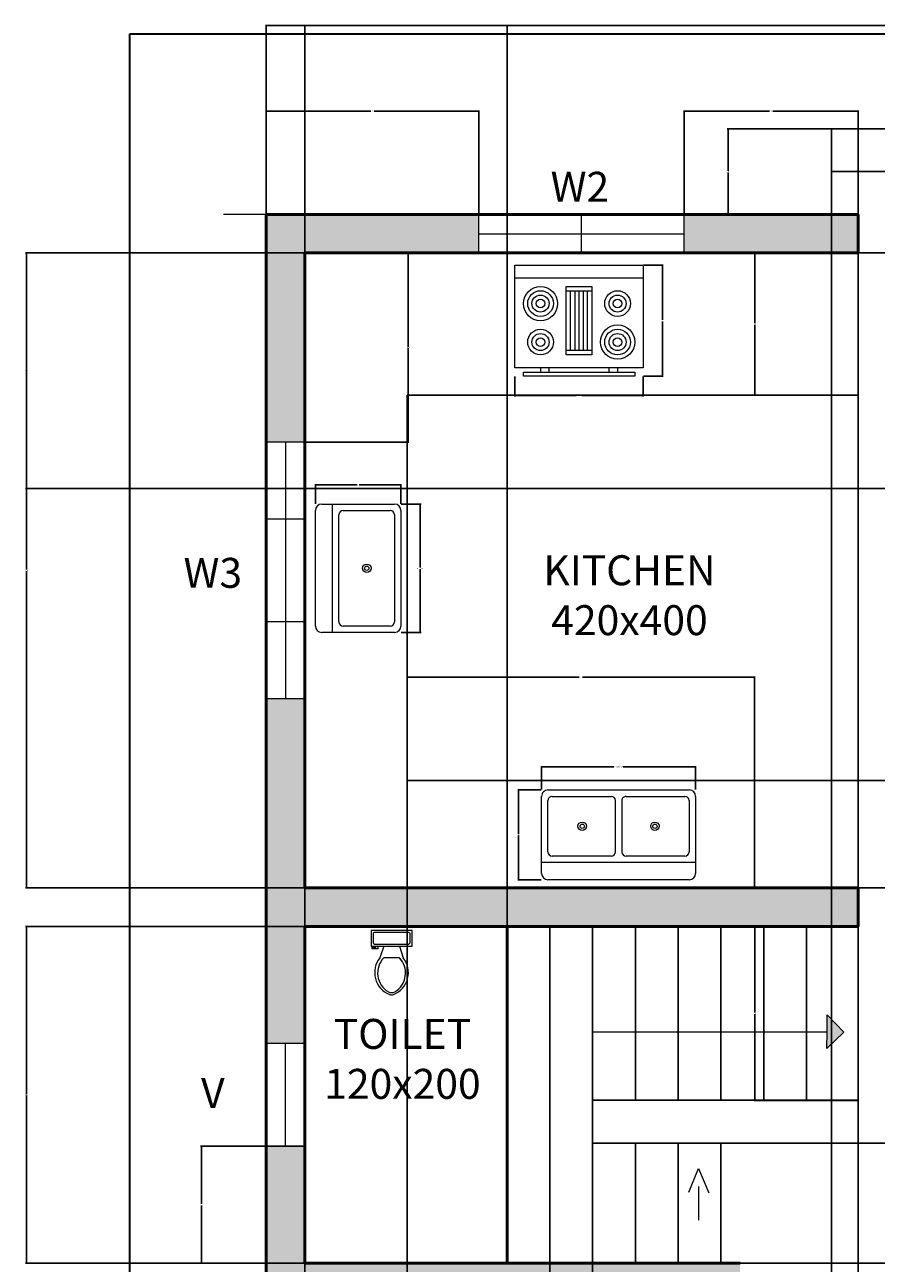
# Model space of a CAD drawing. Units: inches. Extents: x 5191 to 5616, y 7031 to 7539.
# Tile 3 of 4: x 5191 to 5390, y 7250 to 7539. Entities that reach past the tile are written whole.
import ezdxf

# ---------------------------------------------------------------- set-up
doc = ezdxf.new("R2010")
doc.units = ezdxf.units.IN
for name, color, linetype, lineweight in [('A-ANNO-DIMS', 2, 'Continuous', 13), ('A-ANNO-SYMB', 7, 'Continuous', 18), ('A-ANNO-TEXT', 7, 'Continuous', 18), ('A-ANNO-TTLB', 7, 'Continuous', 35), ('A-AREA-IDEN', 7, 'Continuous', 25), ('A-EQPM', 8, 'Continuous', 18), ('A-FLOR-CASE', 8, 'Continuous', 25), ('A-FLOR-FIXT', 9, 'Continuous', 18), ('A-FLOR-STRS', 7, 'Continuous', 25), ('A-GLAZ', 4, 'Continuous', 18), ('A-WALL', 7, 'Continuous', 50)]:
    doc.layers.add(name, color=color, linetype=linetype, lineweight=lineweight)
doc.layers.add('A-WALL-PATT', color=177, linetype='Continuous', lineweight=13, true_color=0x293189)
doc.styles.get("Standard").update_dxf_attribs({"font": 'arial.ttf'})
doc.dimstyles.get("Standard").update_dxf_attribs({"dimtxt": 0.18, "dimasz": 0.18, "dimexe": 0.18, "dimexo": 0.0625, "dimgap": 0.09, "dimtad": 0, "dimtih": 1, "dimtoh": 1, "dimdec": 4, "dimzin": 0, "dimdsep": 46, "dimtxsty": 'Standard', "dimcen": 0.09, "dimadec": 0, "dimazin": 0, "dimtfac": 1, "dimtdec": 4, "dimtofl": 0, "dimtmove": 0, "dimatfit": 3, "dimfxl": 1, "dimtolj": 1, "dimtzin": 0, "dimarcsym": 0})

# ---------------------------------------------------------------- blocks, each defined once
blk = doc.blocks.new('*U2')
for p, q in [((9.5, -6), (9.5, -2)), ((-10, -8.5), (-8, -8.5)), ((-10, -9.5), (-10, -8.5)), ((-7, -9.5), (-10, -9.5)), ((-8, -8.5), (-8, -8)), ((-7, -8), (-7, -9.5)), ((-4, -8), (-6, -14)), ((4, -8), (6, -14)), ((4, -14), (-4, -14))]:
    blk.add_line(p, q)
blk.add_lwpolyline([(10.5, -8), (10.5, 0), (-10.5, 0), (-10.5, -8)], close=True)
for points in [[(-9.5, -2), (-9.5, -6)], [(8.5, -1), (-8.5, -1)], [(-8.5, -7), (8.5, -7)]]:
    blk.add_lwpolyline(points)
for centre, radius, start, end in [((-8.62, -1.88), 0.884, 81.8699, 188.1301), ((-8.62, -6.12), 0.884, 171.8699, 278.1301), ((8.62, -1.88), 0.884, 351.8699, 98.1301), ((8.62, -6.12), 0.884, 261.8699, 8.1301), ((3.52, -21.58), 12.17, 141.46911, 247.97143), ((4.2, -21.82), 11.33, 136.36773, 238.94682), ((-3.52, -21.58), 12.17, 292.02843, 38.53071), ((-4.2, -21.82), 11.33, 301.05301, 43.63209), ((0, -27.88), 4, 245.73182, 294.26817), ((0, -29), 4, 254.86053, 285.13947)]:
    blk.add_arc(centre, radius, start, end)
blk = doc.blocks.new('Range-Oven - 30 in top')
for p, q in [((0, -3), (30, -3)), ((12, -6), (18, -6)), ((13, -20), (13, -6)), ((14, -6), (14, -20)), ((15, -20), (15, -6)), ((16, -6), (16, -20)), ((17, -20), (17, -6)), ((18, -20), (12, -20)), ((6, -24), (6, -25)), ((8, -25), (8, -24)), ((22, -25), (22, -24)), ((24, -24), (24, -25))]:
    blk.add_line(p, q)
for points in [[(0, -24), (0, 0), (30, 0), (30, -24)], [(12, -21), (12, -5), (18, -5), (18, -21)], [(2, -26), (2, -25), (28, -25), (28, -26)]]:
    blk.add_lwpolyline(points, close=True)
for centre, radius in [((6, -9), 4), ((6, -9), 3), ((6, -9), 2), ((6, -9), 1), ((24, -9), 3), ((24, -9), 2), ((24, -9), 1), ((24, -18), 4), ((6, -18), 3), ((6, -18), 2), ((6, -18), 1), ((24, -18), 3), ((24, -18), 2), ((24, -18), 1)]:
    blk.add_circle(centre, radius)
blk = doc.blocks.new('Sink-double - 36 in top')
for p, q in [((-18, -4), (18, -4)), ((-0.75, -18.5), (-0.75, -6.5)), ((0.75, -6.5), (0.75, -18.5))]:
    blk.add_line(p, q)
for points in [[(-16.5, 0), (16.5, 0)], [(-18, -19.5), (-18, -1.5)], [(18, -1.5), (18, -19.5)], [(-15.5, -5.5), (-1.75, -5.5)], [(1.75, -5.5), (15.5, -5.5)], [(-16.5, -18.5), (-16.5, -6.5)], [(16.5, -6.5), (16.5, -18.5)], [(-1.75, -19.5), (-15.5, -19.5)], [(15.5, -19.5), (1.75, -19.5)], [(16.5, -21), (-16.5, -21)]]:
    blk.add_lwpolyline(points)
for centre, radius in [((-8.5, -12.5), 1), ((8.5, -12.5), 1), ((-8.5, -12.5), 0.5), ((8.5, -12.5), 0.5)]:
    blk.add_circle(centre, radius)
for centre, radius, start, end in [((-16.5, -1.5), 1.5, 90, 180), ((16.5, -1.5), 1.5, 0, 90), ((-15.5, -6.5), 1, 90, 180), ((-1.75, -6.5), 1, 0, 90), ((1.75, -6.5), 1, 90, 180), ((15.5, -6.5), 1, 0, 90), ((-16.5, -19.5), 1.5, 180, 270), ((-15.5, -18.5), 1, 180, 270), ((-1.75, -18.5), 1, 270, 0), ((1.75, -18.5), 1, 180, 270), ((15.5, -18.5), 1, 270, 0), ((16.5, -19.5), 1.5, 270, 0)]:
    blk.add_arc(centre, radius, start, end)
blk = doc.blocks.new('Sink-single - 30 in top')
blk.add_line((-15, -3.999996), (15, -3.999996))
for points in [[(-13.5, 0), (13.5, 0)], [(-15, -18.499996), (-15, -1.5)], [(15, -1.5), (15, -18.499996)], [(-12.5, -5.499996), (12.5, -5.499996)], [(-13.5, -17.499996), (-13.5, -6.499996)], [(13.5, -6.499996), (13.5, -17.499996)], [(13.5, -19.999996), (-13.5, -19.999996)], [(12.5, -18.499996), (-12.5, -18.499996)]]:
    blk.add_lwpolyline(points)
for radius in [1, 0.5]:
    blk.add_circle((0, -11.999996), radius)
for centre, radius, start, end in [((-13.5, -1.5), 1.5, 90, 180), ((13.5, -1.5), 1.5, 0, 90), ((-12.5, -6.499996), 1, 90, 180), ((12.5, -6.499996), 1, 0, 90), ((-13.5, -18.499996), 1.5, 180, 270), ((-12.5, -17.499996), 1, 180, 270), ((12.5, -17.499996), 1, 270, 0), ((13.5, -18.499996), 1.5, 270, 0)]:
    blk.add_arc(centre, radius, start, end)
blk = doc.blocks.new('WIN-W2-48IN')
for p, q in [((0, 0), (0, 9)), ((24, 0), (24, 9)), ((48, 0), (48, 9)), ((0, 4.5), (48, 4.5))]:
    blk.add_line(p, q)
blk = doc.blocks.new('WIN-W3-60IN')
for p, q in [((9, 60), (0, 60)), ((4.5, 60), (4.5, 0)), ((9, 42), (0, 42)), ((9, 18), (0, 18)), ((9, 0), (0, 0))]:
    blk.add_line(p, q)
blk = doc.blocks.new('VENT-24IN')
for p, q in [((0, 0), (0, 9)), ((24, 0), (24, 9)), ((0, 4.5), (24, 4.5))]:
    blk.add_line(p, q)
blk = doc.blocks.new('*D25')
at = {"layer": 'A-ANNO-DIMS', "color": 0, "lineweight": -2, "transparency": 16777216}
for p, q in [((5305.74, 7456.87), (5305.74, 7452.25)), ((5335.74, 7456.87), (5335.74, 7452.25)), ((5305.92, 7452.43), (5320.05, 7452.43)), ((5335.56, 7452.43), (5321.44, 7452.43))]:
    blk.add_line(p, q, dxfattribs=at)
at = {"layer": 'A-ANNO-DIMS', "color": 0, "transparency": 16777216}
for points in [[(5305.92, 7452.46), (5305.92, 7452.4), (5305.74, 7452.43)], [(5335.56, 7452.46), (5335.56, 7452.4), (5335.74, 7452.43)]]:
    blk.add_solid(points, dxfattribs=at)
at = {"layer": 'Defpoints', "color": 0, "transparency": 16777216}
for p in [(5305.74, 7456.93), (5335.74, 7456.93), (5335.74, 7452.43)]:
    blk.add_point(p, dxfattribs=at)
at = {"layer": 'A-ANNO-DIMS', "color": 0, "transparency": 16777216, "insert": (5320.74, 7452.43), "char_height": 0.18, "attachment_point": 5}
blk.add_mtext('\\A1;RANGE 30', dxfattribs=at)
blk = doc.blocks.new('*D26')
at = {"layer": 'A-ANNO-DIMS', "color": 0, "lineweight": -2, "transparency": 16777216}
for p, q in [((5335.81, 7482.93), (5340.42, 7482.93)), ((5340.24, 7482.75), (5340.24, 7470.12)), ((5340.24, 7457.11), (5340.24, 7469.75)), ((5335.81, 7456.93), (5340.42, 7456.93))]:
    blk.add_line(p, q, dxfattribs=at)
at = {"layer": 'A-ANNO-DIMS', "color": 0, "transparency": 16777216}
for points in [[(5340.21, 7482.75), (5340.27, 7482.75), (5340.24, 7482.93)], [(5340.21, 7457.11), (5340.27, 7457.11), (5340.24, 7456.93)]]:
    blk.add_solid(points, dxfattribs=at)
at = {"layer": 'Defpoints', "color": 0, "transparency": 16777216}
for p in [(5335.74, 7482.93), (5340.24, 7482.93), (5335.74, 7456.93)]:
    blk.add_point(p, dxfattribs=at)
at = {"layer": 'A-ANNO-DIMS', "color": 0, "transparency": 16777216, "insert": (5340.24, 7469.93), "char_height": 0.18, "attachment_point": 5}
blk.add_mtext('\\A1;26', dxfattribs=at)
blk = doc.blocks.new('*D27')
at = {"layer": 'A-ANNO-DIMS', "color": 0, "lineweight": -2, "transparency": 16777216}
for p, q in [((5311.98, 7360.31), (5311.98, 7365.83)), ((5312.16, 7365.65), (5328.89, 7365.65)), ((5347.8, 7365.65), (5331.08, 7365.65)), ((5347.98, 7360.31), (5347.98, 7365.83))]:
    blk.add_line(p, q, dxfattribs=at)
at = {"layer": 'A-ANNO-DIMS', "color": 0, "transparency": 16777216}
for points in [[(5312.16, 7365.68), (5312.16, 7365.62), (5311.98, 7365.65)], [(5347.8, 7365.68), (5347.8, 7365.62), (5347.98, 7365.65)]]:
    blk.add_solid(points, dxfattribs=at)
at = {"layer": 'Defpoints', "color": 0, "transparency": 16777216}
for p in [(5311.98, 7365.65), (5311.98, 7360.25), (5347.98, 7360.25)]:
    blk.add_point(p, dxfattribs=at)
at = {"layer": 'A-ANNO-DIMS', "color": 0, "transparency": 16777216, "insert": (5329.98, 7365.65), "char_height": 0.18, "attachment_point": 5}
blk.add_mtext('\\A1;DOUBLE SINK 36', dxfattribs=at)
blk = doc.blocks.new('*D28')
at = {"layer": 'A-ANNO-DIMS', "color": 0, "lineweight": -2, "transparency": 16777216}
for p, q in [((5311.92, 7360.25), (5306.4, 7360.25)), ((5306.58, 7360.07), (5306.58, 7349.93)), ((5306.58, 7339.43), (5306.58, 7349.56)), ((5311.92, 7339.25), (5306.4, 7339.25))]:
    blk.add_line(p, q, dxfattribs=at)
at = {"layer": 'A-ANNO-DIMS', "color": 0, "transparency": 16777216}
for points in [[(5306.55, 7360.07), (5306.61, 7360.07), (5306.58, 7360.25)], [(5306.55, 7339.43), (5306.61, 7339.43), (5306.58, 7339.25)]]:
    blk.add_solid(points, dxfattribs=at)
at = {"layer": 'Defpoints', "color": 0, "transparency": 16777216}
for p in [(5311.98, 7360.25), (5306.58, 7339.25), (5311.98, 7339.25)]:
    blk.add_point(p, dxfattribs=at)
at = {"layer": 'A-ANNO-DIMS', "color": 0, "transparency": 16777216, "insert": (5306.58, 7349.75), "char_height": 0.18, "attachment_point": 5}
blk.add_mtext('\\A1;21', dxfattribs=at)
blk = doc.blocks.new('*D29')
at = {"layer": 'A-ANNO-DIMS', "color": 0, "lineweight": -2, "transparency": 16777216}
for p, q in [((5279.2, 7427.05), (5283.81, 7427.05)), ((5283.63, 7426.87), (5283.63, 7412.24)), ((5283.63, 7397.23), (5283.63, 7411.87)), ((5279.2, 7397.05), (5283.81, 7397.05))]:
    blk.add_line(p, q, dxfattribs=at)
at = {"layer": 'A-ANNO-DIMS', "color": 0, "transparency": 16777216}
for points in [[(5283.6, 7426.87), (5283.66, 7426.87), (5283.63, 7427.05)], [(5283.6, 7397.23), (5283.66, 7397.23), (5283.63, 7397.05)]]:
    blk.add_solid(points, dxfattribs=at)
at = {"layer": 'Defpoints', "color": 0, "transparency": 16777216}
for p in [(5279.13, 7427.05), (5283.63, 7427.05), (5279.13, 7397.05)]:
    blk.add_point(p, dxfattribs=at)
at = {"layer": 'A-ANNO-DIMS', "color": 0, "transparency": 16777216, "insert": (5283.63, 7412.05), "char_height": 0.18, "attachment_point": 5}
blk.add_mtext('\\A1;SINGLE SINK 30', dxfattribs=at)
blk = doc.blocks.new('*D30')
at = {"layer": 'A-ANNO-DIMS', "color": 0, "lineweight": -2, "transparency": 16777216}
for p, q in [((5259.13, 7427.12), (5259.13, 7431.73)), ((5259.31, 7431.55), (5268.91, 7431.55)), ((5278.95, 7431.55), (5269.35, 7431.55)), ((5279.13, 7427.12), (5279.13, 7431.73))]:
    blk.add_line(p, q, dxfattribs=at)
at = {"layer": 'A-ANNO-DIMS', "color": 0, "transparency": 16777216}
for points in [[(5259.31, 7431.58), (5259.31, 7431.52), (5259.13, 7431.55)], [(5278.95, 7431.58), (5278.95, 7431.52), (5279.13, 7431.55)]]:
    blk.add_solid(points, dxfattribs=at)
at = {"layer": 'Defpoints', "color": 0, "transparency": 16777216}
for p in [(5259.13, 7431.55), (5259.13, 7427.05), (5279.13, 7427.05)]:
    blk.add_point(p, dxfattribs=at)
at = {"layer": 'A-ANNO-DIMS', "color": 0, "transparency": 16777216, "insert": (5269.13, 7431.55), "char_height": 0.18, "attachment_point": 5}
blk.add_mtext('\\A1;20', dxfattribs=at)
blk = doc.blocks.new('*D31')
at = {"layer": 'A-ANNO-DIMS', "color": 0, "lineweight": -2, "transparency": 16777216}
for p, q in [((5247.63, 7494.84), (5247.63, 7539.1)), ((5247.81, 7538.92), (5402.39, 7538.92)), ((5557.89, 7538.92), (5403.31, 7538.92)), ((5558.07, 7494.84), (5558.07, 7539.1))]:
    blk.add_line(p, q, dxfattribs=at)
at = {"layer": 'A-ANNO-DIMS', "color": 0, "transparency": 16777216}
for points in [[(5247.81, 7538.95), (5247.81, 7538.89), (5247.63, 7538.92)], [(5557.89, 7538.95), (5557.89, 7538.89), (5558.07, 7538.92)]]:
    blk.add_solid(points, dxfattribs=at)
at = {"layer": 'Defpoints', "color": 0, "transparency": 16777216}
for p in [(5558.07, 7538.92), (5247.63, 7494.77), (5558.07, 7494.77)]:
    blk.add_point(p, dxfattribs=at)
at = {"layer": 'A-ANNO-DIMS', "color": 0, "transparency": 16777216, "insert": (5402.85, 7538.92), "char_height": 0.18, "attachment_point": 5}
blk.add_mtext('\\A1;310.44', dxfattribs=at)
blk = doc.blocks.new('*D37')
at = {"layer": 'A-ANNO-DIMS', "color": 0, "lineweight": -2, "transparency": 16777216}
for p, q in [((5379.65, 7514.77), (5355.38, 7514.77)), ((5355.56, 7514.59), (5355.56, 7504.96)), ((5355.56, 7494.95), (5355.56, 7504.59)), ((5379.65, 7494.77), (5355.38, 7494.77))]:
    blk.add_line(p, q, dxfattribs=at)
at = {"layer": 'A-ANNO-DIMS', "color": 0, "transparency": 16777216}
for points in [[(5355.53, 7514.59), (5355.59, 7514.59), (5355.56, 7514.77)], [(5355.53, 7494.95), (5355.59, 7494.95), (5355.56, 7494.77)]]:
    blk.add_solid(points, dxfattribs=at)
at = {"layer": 'Defpoints', "color": 0, "transparency": 16777216}
for p in [(5355.56, 7514.77), (5379.71, 7514.77), (5379.71, 7494.77)]:
    blk.add_point(p, dxfattribs=at)
at = {"layer": 'A-ANNO-DIMS', "color": 0, "transparency": 16777216, "insert": (5355.56, 7504.77), "char_height": 0.18, "attachment_point": 5}
blk.add_mtext('\\A1;20', dxfattribs=at)
blk = doc.blocks.new('*D38')
at = {"layer": 'A-ANNO-DIMS', "color": 0, "lineweight": -2, "transparency": 16777216}
for p, q in [((5379.71, 7504.71), (5379.71, 7030.92)), ((5428.18, 7504.71), (5428.18, 7030.92)), ((5379.89, 7031.1), (5403.55, 7031.1)), ((5428, 7031.1), (5404.34, 7031.1))]:
    blk.add_line(p, q, dxfattribs=at)
at = {"layer": 'A-ANNO-DIMS', "color": 0, "transparency": 16777216}
for points in [[(5379.89, 7031.13), (5379.89, 7031.07), (5379.71, 7031.1)], [(5428, 7031.13), (5428, 7031.07), (5428.18, 7031.1)]]:
    blk.add_solid(points, dxfattribs=at)
at = {"layer": 'Defpoints', "color": 0, "transparency": 16777216}
for p in [(5379.71, 7504.77), (5428.18, 7504.77), (5428.18, 7031.1)]:
    blk.add_point(p, dxfattribs=at)
at = {"layer": 'A-ANNO-DIMS', "color": 0, "transparency": 16777216, "insert": (5403.95, 7031.1), "char_height": 0.18, "attachment_point": 5}
blk.add_mtext('\\A1;48.47', dxfattribs=at)
blk = doc.blocks.new('*D40')
at = {"layer": 'A-ANNO-DIMS', "color": 0, "lineweight": -2, "transparency": 16777216}
for p, q in [((5256.57, 7328.33), (5191.41, 7328.33)), ((5191.59, 7328.15), (5191.59, 7289.16)), ((5191.59, 7249.79), (5191.59, 7288.79)), ((5256.57, 7249.61), (5191.41, 7249.61))]:
    blk.add_line(p, q, dxfattribs=at)
at = {"layer": 'A-ANNO-DIMS', "color": 0, "transparency": 16777216}
for points in [[(5191.56, 7328.15), (5191.62, 7328.15), (5191.59, 7328.33)], [(5191.56, 7249.79), (5191.62, 7249.79), (5191.59, 7249.61)]]:
    blk.add_solid(points, dxfattribs=at)
at = {"layer": 'Defpoints', "color": 0, "transparency": 16777216}
for p in [(5191.59, 7328.33), (5256.63, 7328.33), (5256.63, 7249.61)]:
    blk.add_point(p, dxfattribs=at)
at = {"layer": 'A-ANNO-DIMS', "color": 0, "transparency": 16777216, "insert": (5191.59, 7288.97), "char_height": 0.18, "attachment_point": 5}
blk.add_mtext('\\A1;78.72', dxfattribs=at)
blk = doc.blocks.new('*D41')
at = {"layer": 'A-ANNO-DIMS', "color": 0, "lineweight": -2, "transparency": 16777216}
for p, q in [((5256.57, 7485.77), (5191.41, 7485.77)), ((5191.59, 7485.59), (5191.59, 7411.74)), ((5191.59, 7337.51), (5191.59, 7411.37)), ((5256.57, 7337.33), (5191.41, 7337.33))]:
    blk.add_line(p, q, dxfattribs=at)
at = {"layer": 'A-ANNO-DIMS', "color": 0, "transparency": 16777216}
for points in [[(5191.56, 7485.59), (5191.62, 7485.59), (5191.59, 7485.77)], [(5191.56, 7337.51), (5191.62, 7337.51), (5191.59, 7337.33)]]:
    blk.add_solid(points, dxfattribs=at)
at = {"layer": 'Defpoints', "color": 0, "transparency": 16777216}
for p in [(5191.59, 7485.77), (5256.63, 7485.77), (5256.63, 7337.33)]:
    blk.add_point(p, dxfattribs=at)
at = {"layer": 'A-ANNO-DIMS', "color": 0, "transparency": 16777216, "insert": (5191.59, 7411.55), "char_height": 0.18, "attachment_point": 5}
blk.add_mtext('\\A1;148.44', dxfattribs=at)
blk = doc.blocks.new('*D47')
at = {"layer": 'A-ANNO-DIMS', "color": 0, "lineweight": -2, "transparency": 16777216}
for p, q in [((5247.63, 7494.84), (5247.63, 7519.1)), ((5247.81, 7518.92), (5272.07, 7518.92)), ((5297.13, 7518.92), (5272.87, 7518.92)), ((5297.31, 7494.84), (5297.31, 7519.1))]:
    blk.add_line(p, q, dxfattribs=at)
at = {"layer": 'A-ANNO-DIMS', "color": 0, "transparency": 16777216}
for points in [[(5247.81, 7518.95), (5247.81, 7518.89), (5247.63, 7518.92)], [(5297.13, 7518.95), (5297.13, 7518.89), (5297.31, 7518.92)]]:
    blk.add_solid(points, dxfattribs=at)
at = {"layer": 'Defpoints', "color": 0, "transparency": 16777216}
for p in [(5297.31, 7518.92), (5247.63, 7494.77), (5297.31, 7494.77)]:
    blk.add_point(p, dxfattribs=at)
at = {"layer": 'A-ANNO-DIMS', "color": 0, "transparency": 16777216, "insert": (5272.47, 7518.92), "char_height": 0.18, "attachment_point": 5}
blk.add_mtext('\\A1;49.68', dxfattribs=at)
blk = doc.blocks.new('*D48')
at = {"layer": 'A-ANNO-DIMS', "color": 0, "lineweight": -2, "transparency": 16777216}
for p, q in [((5345.31, 7494.84), (5345.31, 7519.1)), ((5345.49, 7518.92), (5365.25, 7518.92)), ((5385.81, 7518.92), (5366.05, 7518.92)), ((5385.99, 7494.84), (5385.99, 7519.1))]:
    blk.add_line(p, q, dxfattribs=at)
at = {"layer": 'A-ANNO-DIMS', "color": 0, "transparency": 16777216}
for points in [[(5345.49, 7518.95), (5345.49, 7518.89), (5345.31, 7518.92)], [(5385.81, 7518.95), (5385.81, 7518.89), (5385.99, 7518.92)]]:
    blk.add_solid(points, dxfattribs=at)
at = {"layer": 'Defpoints', "color": 0, "transparency": 16777216}
for p in [(5385.99, 7518.92), (5345.31, 7494.77), (5385.99, 7494.77)]:
    blk.add_point(p, dxfattribs=at)
at = {"layer": 'A-ANNO-DIMS', "color": 0, "transparency": 16777216, "insert": (5365.65, 7518.92), "char_height": 0.18, "attachment_point": 5}
blk.add_mtext('\\A1;40.68', dxfattribs=at)
blk = doc.blocks.new('*D49')
at = {"layer": 'A-ANNO-DIMS', "color": 0, "lineweight": -2, "transparency": 16777216}
for p, q in [((5385.99, 7494.71), (5385.99, 7030.92)), ((5421.99, 7494.71), (5421.99, 7030.92)), ((5386.17, 7031.1), (5403.77, 7031.1)), ((5421.81, 7031.1), (5404.21, 7031.1))]:
    blk.add_line(p, q, dxfattribs=at)
at = {"layer": 'A-ANNO-DIMS', "color": 0, "transparency": 16777216}
for points in [[(5386.17, 7031.13), (5386.17, 7031.07), (5385.99, 7031.1)], [(5421.81, 7031.13), (5421.81, 7031.07), (5421.99, 7031.1)]]:
    blk.add_solid(points, dxfattribs=at)
at = {"layer": 'Defpoints', "color": 0, "transparency": 16777216}
for p in [(5385.99, 7494.77), (5421.99, 7494.77), (5421.99, 7031.1)]:
    blk.add_point(p, dxfattribs=at)
at = {"layer": 'A-ANNO-DIMS', "color": 0, "transparency": 16777216, "insert": (5403.99, 7031.1), "char_height": 0.18, "attachment_point": 5}
blk.add_mtext('\\A1;36', dxfattribs=at)
blk = doc.blocks.new('*D53')
at = {"layer": 'A-ANNO-DIMS', "color": 0, "lineweight": -2, "transparency": 16777216}
for p, q in [((5256.63, 7249.68), (5256.63, 7539.1)), ((5256.81, 7538.92), (5279.87, 7538.92)), ((5303.73, 7538.92), (5280.67, 7538.92)), ((5303.91, 7249.68), (5303.91, 7539.1))]:
    blk.add_line(p, q, dxfattribs=at)
at = {"layer": 'A-ANNO-DIMS', "color": 0, "transparency": 16777216}
for points in [[(5256.81, 7538.95), (5256.81, 7538.89), (5256.63, 7538.92)], [(5303.73, 7538.95), (5303.73, 7538.89), (5303.91, 7538.92)]]:
    blk.add_solid(points, dxfattribs=at)
at = {"layer": 'Defpoints', "color": 0, "transparency": 16777216}
for p in [(5303.91, 7538.92), (5256.63, 7249.61), (5303.91, 7249.61)]:
    blk.add_point(p, dxfattribs=at)
at = {"layer": 'A-ANNO-DIMS', "color": 0, "transparency": 16777216, "insert": (5280.27, 7538.92), "char_height": 0.18, "attachment_point": 5}
blk.add_mtext('\\A1;47.28', dxfattribs=at)
blk = doc.blocks.new('*D55')
at = {"layer": 'A-ANNO-DIMS', "color": 0, "lineweight": -2, "transparency": 16777216}
for p, q in [((5430.93, 7485.77), (5191.41, 7485.77)), ((5191.59, 7485.59), (5191.59, 7458.42)), ((5191.59, 7430.87), (5191.59, 7458.05)), ((5430.93, 7430.69), (5191.41, 7430.69))]:
    blk.add_line(p, q, dxfattribs=at)
at = {"layer": 'A-ANNO-DIMS', "color": 0, "transparency": 16777216}
for points in [[(5191.56, 7485.59), (5191.62, 7485.59), (5191.59, 7485.77)], [(5191.56, 7430.87), (5191.62, 7430.87), (5191.59, 7430.69)]]:
    blk.add_solid(points, dxfattribs=at)
at = {"layer": 'Defpoints', "color": 0, "transparency": 16777216}
for p in [(5191.59, 7485.77), (5430.99, 7485.77), (5430.99, 7430.69)]:
    blk.add_point(p, dxfattribs=at)
at = {"layer": 'A-ANNO-DIMS', "color": 0, "transparency": 16777216, "insert": (5191.59, 7458.23), "char_height": 0.18, "attachment_point": 5}
blk.add_mtext('\\A1;55.08', dxfattribs=at)
blk = doc.blocks.new('*D56')
at = {"layer": 'A-ANNO-DIMS', "color": 0, "lineweight": -2, "transparency": 16777216}
for p, q in [((5256.69, 7485.77), (5280.96, 7485.77)), ((5280.78, 7485.59), (5280.78, 7463.84)), ((5280.78, 7441.73), (5280.78, 7463.48)), ((5256.69, 7441.55), (5280.96, 7441.55))]:
    blk.add_line(p, q, dxfattribs=at)
at = {"layer": 'A-ANNO-DIMS', "color": 0, "transparency": 16777216}
for points in [[(5280.75, 7485.59), (5280.81, 7485.59), (5280.78, 7485.77)], [(5280.75, 7441.73), (5280.81, 7441.73), (5280.78, 7441.55)]]:
    blk.add_solid(points, dxfattribs=at)
at = {"layer": 'Defpoints', "color": 0, "transparency": 16777216}
for p in [(5256.63, 7485.77), (5256.63, 7441.55), (5280.78, 7441.55)]:
    blk.add_point(p, dxfattribs=at)
at = {"layer": 'A-ANNO-DIMS', "color": 0, "transparency": 16777216, "insert": (5280.78, 7463.66), "char_height": 0.18, "attachment_point": 5}
blk.add_mtext('\\A1;44.22', dxfattribs=at)
blk = doc.blocks.new('*D57')
at = {"layer": 'A-ANNO-DIMS', "color": 0, "lineweight": -2, "transparency": 16777216}
for p, q in [((5256.57, 7276.97), (5232.3, 7276.97)), ((5232.48, 7276.79), (5232.48, 7263.48)), ((5232.48, 7249.79), (5232.48, 7263.11)), ((5256.57, 7249.61), (5232.3, 7249.61))]:
    blk.add_line(p, q, dxfattribs=at)
at = {"layer": 'A-ANNO-DIMS', "color": 0, "transparency": 16777216}
for points in [[(5232.45, 7276.79), (5232.51, 7276.79), (5232.48, 7276.97)], [(5232.45, 7249.79), (5232.51, 7249.79), (5232.48, 7249.61)]]:
    blk.add_solid(points, dxfattribs=at)
at = {"layer": 'Defpoints', "color": 0, "transparency": 16777216}
for p in [(5232.48, 7276.97), (5256.63, 7276.97), (5256.63, 7249.61)]:
    blk.add_point(p, dxfattribs=at)
at = {"layer": 'A-ANNO-DIMS', "color": 0, "transparency": 16777216, "insert": (5232.48, 7263.29), "char_height": 0.18, "attachment_point": 5}
blk.add_mtext('\\A1;27.36', dxfattribs=at)
blk = doc.blocks.new('*D59')
at = {"layer": 'A-ANNO-DIMS', "color": 0, "lineweight": -2, "transparency": 16777216}
for p, q in [((5313.91, 7328.27), (5313.91, 7030.92)), ((5323.91, 7328.27), (5323.91, 7030.92)), ((5314.09, 7031.1), (5318.7, 7031.1)), ((5323.73, 7031.1), (5319.12, 7031.1))]:
    blk.add_line(p, q, dxfattribs=at)
at = {"layer": 'A-ANNO-DIMS', "color": 0, "transparency": 16777216}
for points in [[(5314.09, 7031.13), (5314.09, 7031.07), (5313.91, 7031.1)], [(5323.73, 7031.13), (5323.73, 7031.07), (5323.91, 7031.1)]]:
    blk.add_solid(points, dxfattribs=at)
at = {"layer": 'Defpoints', "color": 0, "transparency": 16777216}
for p in [(5313.91, 7328.33), (5323.91, 7328.33), (5323.91, 7031.1)]:
    blk.add_point(p, dxfattribs=at)
at = {"layer": 'A-ANNO-DIMS', "color": 0, "transparency": 16777216, "insert": (5318.91, 7031.1), "char_height": 0.18, "attachment_point": 5}
blk.add_mtext('\\A1;10', dxfattribs=at)
blk = doc.blocks.new('*D60')
at = {"layer": 'A-ANNO-DIMS', "color": 0, "lineweight": -2, "transparency": 16777216}
for p, q in [((5343.97, 7277.69), (5615.71, 7277.69)), ((5615.53, 7277.51), (5615.53, 7263.84)), ((5615.53, 7249.79), (5615.53, 7263.47)), ((5343.97, 7249.61), (5615.71, 7249.61))]:
    blk.add_line(p, q, dxfattribs=at)
at = {"layer": 'A-ANNO-DIMS', "color": 0, "transparency": 16777216}
for points in [[(5615.5, 7277.51), (5615.56, 7277.51), (5615.53, 7277.69)], [(5615.5, 7249.79), (5615.56, 7249.79), (5615.53, 7249.61)]]:
    blk.add_solid(points, dxfattribs=at)
at = {"layer": 'Defpoints', "color": 0, "transparency": 16777216}
for p in [(5343.91, 7277.69), (5615.53, 7277.69), (5343.91, 7249.61)]:
    blk.add_point(p, dxfattribs=at)
at = {"layer": 'A-ANNO-DIMS', "color": 0, "transparency": 16777216, "insert": (5615.53, 7263.65), "char_height": 0.18, "attachment_point": 5}
blk.add_mtext('\\A1;28.08', dxfattribs=at)
blk = doc.blocks.new('*D61')
at = {"layer": 'A-ANNO-DIMS', "color": 0, "lineweight": -2, "transparency": 16777216}
for p, q in [((5385.93, 7485.77), (5361.66, 7485.77)), ((5361.84, 7485.59), (5361.84, 7469.32)), ((5361.84, 7452.69), (5361.84, 7468.96)), ((5385.93, 7452.51), (5361.66, 7452.51))]:
    blk.add_line(p, q, dxfattribs=at)
at = {"layer": 'A-ANNO-DIMS', "color": 0, "transparency": 16777216}
for points in [[(5361.81, 7485.59), (5361.87, 7485.59), (5361.84, 7485.77)], [(5361.81, 7452.69), (5361.87, 7452.69), (5361.84, 7452.51)]]:
    blk.add_solid(points, dxfattribs=at)
at = {"layer": 'Defpoints', "color": 0, "transparency": 16777216}
for p in [(5361.84, 7485.77), (5385.99, 7485.77), (5385.99, 7452.51)]:
    blk.add_point(p, dxfattribs=at)
at = {"layer": 'A-ANNO-DIMS', "color": 0, "transparency": 16777216, "insert": (5361.84, 7469.14), "char_height": 0.18, "attachment_point": 5}
blk.add_mtext('\\A1;33.266', dxfattribs=at)
blk = doc.blocks.new('*D62')
at = {"layer": 'A-ANNO-DIMS', "color": 0, "lineweight": -2, "transparency": 16777216}
for p, q in [((5361.85, 7362.43), (5615.71, 7362.43)), ((5615.53, 7362.25), (5615.53, 7350.06)), ((5615.53, 7337.51), (5615.53, 7349.7)), ((5361.85, 7337.33), (5615.71, 7337.33))]:
    blk.add_line(p, q, dxfattribs=at)
at = {"layer": 'A-ANNO-DIMS', "color": 0, "transparency": 16777216}
for points in [[(5615.5, 7362.25), (5615.56, 7362.25), (5615.53, 7362.43)], [(5615.5, 7337.51), (5615.56, 7337.51), (5615.53, 7337.33)]]:
    blk.add_solid(points, dxfattribs=at)
at = {"layer": 'Defpoints', "color": 0, "transparency": 16777216}
for p in [(5361.78, 7362.43), (5615.53, 7362.43), (5361.78, 7337.33)]:
    blk.add_point(p, dxfattribs=at)
at = {"layer": 'A-ANNO-DIMS', "color": 0, "transparency": 16777216, "insert": (5615.53, 7349.88), "char_height": 0.18, "attachment_point": 5}
blk.add_mtext('\\A1;25.094', dxfattribs=at)
blk = doc.blocks.new('*D63')
at = {"layer": 'A-ANNO-DIMS', "color": 0, "lineweight": -2, "transparency": 16777216}
for p, q in [((5280.54, 7362.49), (5280.54, 7386.76)), ((5280.72, 7386.58), (5320.77, 7386.58)), ((5361.6, 7386.58), (5321.56, 7386.58)), ((5361.78, 7362.49), (5361.78, 7386.76))]:
    blk.add_line(p, q, dxfattribs=at)
at = {"layer": 'A-ANNO-DIMS', "color": 0, "transparency": 16777216}
for points in [[(5280.72, 7386.61), (5280.72, 7386.55), (5280.54, 7386.58)], [(5361.6, 7386.61), (5361.6, 7386.55), (5361.78, 7386.58)]]:
    blk.add_solid(points, dxfattribs=at)
at = {"layer": 'Defpoints', "color": 0, "transparency": 16777216}
for p in [(5361.78, 7386.58), (5280.54, 7362.43), (5361.78, 7362.43)]:
    blk.add_point(p, dxfattribs=at)
at = {"layer": 'A-ANNO-DIMS', "color": 0, "transparency": 16777216, "insert": (5321.16, 7386.58), "char_height": 0.18, "attachment_point": 5}
blk.add_mtext('\\A1;81.24', dxfattribs=at)
blk = doc.blocks.new('*D64')
at = {"layer": 'A-ANNO-DIMS', "color": 0, "lineweight": -2, "transparency": 16777216}
for p, q in [((5256.63, 7485.71), (5256.63, 7030.92)), ((5280.54, 7452.44), (5280.54, 7030.92)), ((5256.81, 7031.1), (5268.12, 7031.1)), ((5280.36, 7031.1), (5269.05, 7031.1))]:
    blk.add_line(p, q, dxfattribs=at)
at = {"layer": 'A-ANNO-DIMS', "color": 0, "transparency": 16777216}
for points in [[(5256.81, 7031.13), (5256.81, 7031.07), (5256.63, 7031.1)], [(5280.36, 7031.13), (5280.36, 7031.07), (5280.54, 7031.1)]]:
    blk.add_solid(points, dxfattribs=at)
at = {"layer": 'Defpoints', "color": 0, "transparency": 16777216}
for p in [(5256.63, 7485.77), (5280.54, 7452.51), (5280.54, 7031.1)]:
    blk.add_point(p, dxfattribs=at)
at = {"layer": 'A-ANNO-DIMS', "color": 0, "transparency": 16777216, "insert": (5268.59, 7031.1), "char_height": 0.18, "attachment_point": 5}
blk.add_mtext('\\A1;23.913', dxfattribs=at)
blk = doc.blocks.new('*D67')
at = {"layer": 'A-ANNO-DIMS', "color": 0, "lineweight": -2, "transparency": 16777216}
for p, q in [((5385.93, 7328.33), (5361.66, 7328.33)), ((5361.84, 7328.15), (5361.84, 7308.2)), ((5361.84, 7287.87), (5361.84, 7307.83)), ((5385.93, 7287.69), (5361.66, 7287.69))]:
    blk.add_line(p, q, dxfattribs=at)
at = {"layer": 'A-ANNO-DIMS', "color": 0, "transparency": 16777216}
for points in [[(5361.81, 7328.15), (5361.87, 7328.15), (5361.84, 7328.33)], [(5361.81, 7287.87), (5361.87, 7287.87), (5361.84, 7287.69)]]:
    blk.add_solid(points, dxfattribs=at)
at = {"layer": 'Defpoints', "color": 0, "transparency": 16777216}
for p in [(5361.84, 7328.33), (5385.99, 7328.33), (5385.99, 7287.69)]:
    blk.add_point(p, dxfattribs=at)
at = {"layer": 'A-ANNO-DIMS', "color": 0, "transparency": 16777216, "insert": (5361.84, 7308.01), "char_height": 0.18, "attachment_point": 5}
blk.add_mtext('\\A1;40.64', dxfattribs=at)

msp = doc.modelspace()

# ---------------------------------------------------------------- hatches: boundary and pattern name
at = {"layer": 'A-ANNO-SYMB'}
h = msp.add_hatch(color=256, dxfattribs=at)
h.dxf.hatch_style = 1
h.paths.add_polyline_path([(5382.6256, 7303.6347), (5378.7063, 7307.7065), (5378.7063, 7303.6923), (5378.6455, 7299.8038)])
at = {"layer": 'A-WALL-PATT'}
h = msp.add_hatch(color=256, dxfattribs=at)
h.dxf.hatch_style = 1
h.paths.add_polyline_path([(5297.311, 7494.7733), (5247.631, 7494.7733), (5247.631, 7441.5533), (5256.631, 7441.5533), (5256.631, 7485.7733), (5297.311, 7485.7733)])
h.paths.add_polyline_path([(5503.471, 7430.6933), (5503.471, 7461.7733), (5494.471, 7461.7733), (5494.471, 7430.6933), (5430.991, 7430.6933), (5430.991, 7485.7733), (5450.731, 7485.7733), (5450.731, 7494.7733), (5421.991, 7494.7733), (5421.991, 7485.7733), (5421.991, 7337.3333), (5421.991, 7328.3333), (5430.991, 7328.3333), (5430.991, 7337.3333), (5430.991, 7421.6933), (5503.471, 7421.6933)])
h.paths.add_polyline_path([(5385.991, 7494.7733), (5345.311, 7494.7733), (5345.311, 7485.7733), (5385.991, 7485.7733)])
h.paths.add_polyline_path([(5558.071, 7494.7733), (5474.731, 7494.7733), (5474.731, 7485.7733), (5494.471, 7485.7733), (5503.471, 7485.7733), (5549.071, 7485.7733), (5549.071, 7397.3333), (5558.071, 7397.3333)])
h.paths.add_polyline_path([(5385.991, 7337.3333), (5256.631, 7337.3333), (5256.631, 7381.5533), (5247.631, 7381.5533), (5247.631, 7337.3333), (5247.631, 7328.3333), (5247.631, 7300.9733), (5256.631, 7300.9733), (5256.631, 7328.3333), (5385.991, 7328.3333)])
h.paths.add_polyline_path([(5358.391, 7249.6133), (5303.911, 7249.6133), (5256.631, 7249.6133), (5256.631, 7276.9733), (5247.631, 7276.9733), (5247.631, 7249.6133), (5247.631, 7240.6133), (5247.631, 7207.6133), (5256.631, 7207.6133), (5256.631, 7240.6133), (5303.911, 7240.6133), (5358.391, 7240.6133)])
h.paths.add_polyline_path([(5256.631, 7114.6133), (5256.631, 7147.6133), (5247.631, 7147.6133), (5247.631, 7114.6133), (5247.631, 7105.6133), (5247.631, 7087.6133), (5301.511, 7087.6133), (5301.511, 7096.6133), (5256.631, 7096.6133)])
h.paths.add_polyline_path([(5403.391, 7105.6133), (5403.391, 7114.6133), (5403.391, 7134.8933), (5412.4598, 7134.8933), (5412.4598, 7143.8933), (5403.391, 7143.8933), (5403.391, 7249.6133), (5394.391, 7249.6133), (5394.391, 7143.8933), (5394.391, 7134.8933), (5394.391, 7114.6133), (5394.391, 7096.6133), (5349.511, 7096.6133), (5349.511, 7087.6133), (5403.391, 7087.6133)])
h.paths.add_polyline_path([(5558.071, 7143.8933), (5558.071, 7186.7933), (5549.071, 7186.7933), (5549.071, 7143.8933), (5527.2654, 7143.8933), (5527.2654, 7134.8933), (5558.071, 7134.8933)])
h.paths.add_polyline_path([(5479.2654, 7143.8933), (5448.4598, 7143.8933), (5448.4598, 7134.8933), (5479.2654, 7134.8933)])
h.paths.add_polyline_path([(5558.071, 7337.3333), (5549.071, 7337.3333), (5549.071, 7286.6933), (5421.991, 7286.6933), (5421.991, 7277.6933), (5430.991, 7277.6933), (5549.071, 7277.6933), (5549.071, 7234.7933), (5558.071, 7234.7933), (5558.071, 7277.6933)])

# ---------------------------------------------------------------- linework, layer by layer
at = {"layer": 'A-ANNO-DIMS'}
for q in [(5247.631, 7504.7733), (5237.631, 7494.7733)]:
    msp.add_line((5247.631, 7494.7733), q, dxfattribs=at)
at = {"layer": 'A-ANNO-SYMB'}
for p, q in [((5378.7063, 7303.6923), (5378.7063, 7307.7065)), ((5378.7063, 7307.7065), (5382.6256, 7303.6347)), ((5323.911, 7303.6923), (5378.7063, 7303.6923)), ((5378.6455, 7299.8038), (5378.7063, 7303.6923)), ((5382.6256, 7303.6347), (5378.6455, 7299.8038)), ((5346.4053, 7266.2043), (5348.6533, 7271.7791)), ((5348.6533, 7271.7791), (5351.0678, 7266.0379)), ((5348.7365, 7259.7142), (5348.7365, 7267.5356))]:
    msp.add_line(p, q, dxfattribs=at)
at = {"layer": 'A-ANNO-TTLB'}
msp.add_lwpolyline([(5215.7388, 7536.9841), (5591.3795, 7536.9841), (5591.3795, 7055.2452), (5215.7388, 7055.2452)], close=True, dxfattribs=at)
at = {"layer": 'A-FLOR-CASE'}
for p, q in [((5385.991, 7485.7733), (5385.991, 7452.5072)), ((5385.991, 7452.5072), (5280.5439, 7452.5072)), ((5280.5439, 7452.5072), (5280.5439, 7362.4276)), ((5280.5439, 7362.4276), (5361.7831, 7362.4276)), ((5361.7831, 7362.4276), (5361.7831, 7337.3333))]:
    msp.add_line(p, q, dxfattribs=at)
at = {"layer": 'A-FLOR-STRS'}
for p, q in [((5379.7136, 7494.7733), (5379.7136, 7514.7733)), ((5379.7136, 7514.7733), (5428.1805, 7514.7733)), ((5379.7136, 7504.7733), (5428.1805, 7504.7733)), ((5313.911, 7249.6133), (5313.911, 7328.3333)), ((5313.911, 7287.6933), (5313.911, 7328.3333)), ((5323.911, 7287.6933), (5323.911, 7328.3333)), ((5333.911, 7287.6933), (5333.911, 7328.3333)), ((5343.911, 7287.6933), (5343.911, 7328.3333)), ((5353.911, 7287.6933), (5353.911, 7328.3333)), ((5363.911, 7287.6933), (5363.911, 7328.3333)), ((5373.911, 7287.6933), (5373.911, 7328.3333)), ((5385.991, 7328.3333), (5385.991, 7287.6933)), ((5385.991, 7287.6933), (5323.911, 7287.6933)), ((5323.911, 7287.6933), (5323.911, 7277.6933)), ((5313.911, 7249.6133), (5313.911, 7277.6933)), ((5313.911, 7249.6133), (5313.911, 7277.6933)), ((5385.991, 7277.6933), (5323.911, 7277.6933)), ((5323.911, 7249.6133), (5323.911, 7277.6933)), ((5333.911, 7249.6133), (5333.911, 7277.6933)), ((5343.911, 7249.6133), (5343.911, 7277.6933)), ((5353.911, 7249.6133), (5353.911, 7277.6933))]:
    msp.add_line(p, q, dxfattribs=at)
at = {"layer": 'A-WALL'}
for p, q in [((5247.631, 7494.7733), (5247.631, 7337.3333)), ((5247.631, 7494.7733), (5385.991, 7494.7733)), ((5385.991, 7485.7733), (5385.991, 7494.7733)), ((5256.631, 7485.7733), (5256.631, 7337.3333)), ((5256.631, 7485.7733), (5385.991, 7485.7733)), ((5247.631, 7337.3333), (5247.631, 7328.3333)), ((5256.631, 7337.3333), (5385.991, 7337.3333)), ((5385.991, 7337.3333), (5385.991, 7328.3333)), ((5247.631, 7328.3333), (5247.631, 7249.6133)), ((5256.631, 7328.3333), (5385.991, 7328.3333)), ((5256.631, 7328.3333), (5256.631, 7249.6133)), ((5303.911, 7249.6133), (5303.911, 7328.3333)), ((5247.631, 7249.6133), (5247.631, 7240.6133)), ((5256.631, 7249.6133), (5303.911, 7249.6133)), ((5303.911, 7249.6133), (5358.391, 7249.6133))]:
    msp.add_line(p, q, dxfattribs=at)

# ---------------------------------------------------------------- block references
at = {"layer": 'A-EQPM'}
msp.add_blockref('Range-Oven - 30 in top', (5305.7444, 7482.9338), dxfattribs=at)
at = {"layer": 'A-FLOR-FIXT'}
for name, p, rotation in [('Sink-single - 30 in top', (5259.1327, 7412.0549), 90), ('Sink-double - 36 in top', (5329.9847, 7339.2452), 180)]:
    msp.add_blockref(name, p, dxfattribs=dict(at, rotation=rotation))
at = {"layer": 'A-FLOR-FIXT', "xscale": 0.4558429364465041, "yscale": 0.4558429364465041, "zscale": 0.4558429364465041}
msp.add_blockref('*U2', (5276.9276, 7327.4024), dxfattribs=at)
at = {"layer": 'A-GLAZ'}
for name, p in [('WIN-W2-48IN', (5297.311, 7485.773)), ('WIN-W3-60IN', (5247.631, 7381.553))]:
    msp.add_blockref(name, p, dxfattribs=at)
at = {"layer": 'A-GLAZ', "rotation": 89.99999999999477}
msp.add_blockref('VENT-24IN', (5256.6313, 7276.9733), dxfattribs=at)

# ---------------------------------------------------------------- texts
at = {"layer": 'A-ANNO-TEXT', "char_height": 7, "attachment_point": 1}
for s, insert in [('\\pxqc;W2', (5306.0933, 7504.7374)), ('\\pxqc;W3', (5220.3074, 7414.4898)), ('\\pxqc;V', (5220.3074, 7292.8892))]:
    msp.add_mtext_dynamic_manual_height_columns(s, width=29.703042, gutter_width=12.5, heights=[0], dxfattribs=dict(at, insert=insert))
at = {"layer": 'A-AREA-IDEN', "char_height": 7, "attachment_point": 1}
for s, width, insert in [('\\pxqc;{\\fArial|b1|i0|c0|p34;KITCHEN\\P420x400}', 101.484863, (5281.786, 7415.0974)), ('\\pxqc;{\\fArial|b1|i0|c0|p34;TOILET\\P120x200}', 38.465233, (5260.2407, 7306.7129))]:
    msp.add_mtext_dynamic_manual_height_columns(s, width=width, gutter_width=12.5, heights=[0], dxfattribs=dict(at, insert=insert))

# ---------------------------------------------------------------- dimensions: what is measured, and where the dimension line sits
at = {"layer": 'A-ANNO-DIMS'}
for base, p1, p2, override, picture, middle in [((5558.071, 7538.9233), (5247.631, 7494.7733), (5558.071, 7494.7733), {"dimdec": 2, "dimlfac": 1, "dimrnd": 0, "dimzin": 0, "dimdsep": 46, "dimlunit": 2}, '*D31', (5402.851, 7538.9233)), ((5303.911, 7538.9233), (5256.631, 7249.6133), (5303.911, 7249.6133), {"dimdec": 2, "dimlfac": 1, "dimrnd": 0, "dimzin": 0, "dimdsep": 46, "dimlunit": 2}, '*D53', (5280.271, 7538.9233)), ((5297.311, 7518.9233), (5247.631, 7494.7733), (5297.311, 7494.7733), {"dimdec": 2, "dimlfac": 1, "dimrnd": 0, "dimzin": 0, "dimdsep": 46, "dimlunit": 2}, '*D47', (5272.471, 7518.9233)), ((5385.991, 7518.9233), (5345.311, 7494.7733), (5385.991, 7494.7733), {"dimdec": 2, "dimlfac": 1, "dimrnd": 0, "dimzin": 0, "dimdsep": 46, "dimlunit": 2}, '*D48', (5365.651, 7518.9233)), ((5428.1805, 7031.0952), (5379.7136, 7504.7733), (5428.1805, 7504.7733), {"dimdec": 2, "dimlfac": 1, "dimrnd": 0, "dimzin": 0, "dimdsep": 46, "dimlunit": 2}, '*D38', (5403.947, 7031.0952)), ((5421.991, 7031.0952), (5385.991, 7494.7733), (5421.991, 7494.7733), {"dimdec": 0, "dimlfac": 1, "dimrnd": 0, "dimzin": 0, "dimdsep": 46, "dimlunit": 2}, '*D49', (5403.991, 7031.0952)), ((5280.5439, 7031.0952), (5256.631, 7485.7733), (5280.5439, 7452.5072), {"dimdec": 3, "dimlfac": 1, "dimrnd": 0, "dimzin": 0, "dimdsep": 46, "dimlunit": 2}, '*D64', (5268.5874, 7031.0952)), ((5361.7831, 7386.5776), (5280.5439, 7362.4276), (5361.7831, 7362.4276), {"dimdec": 2, "dimlfac": 1, "dimrnd": 0, "dimzin": 0, "dimdsep": 46, "dimlunit": 2}, '*D63', (5321.1635, 7386.5776)), ((5323.911, 7031.0952), (5313.911, 7328.3333), (5323.911, 7328.3333), {"dimdec": 0, "dimlfac": 1, "dimrnd": 0, "dimzin": 0, "dimdsep": 46, "dimlunit": 2}, '*D59', (5318.911, 7031.0952))]:
    dim = msp.add_linear_dim(base=base, p1=p1, p2=p2, dimstyle='Standard', override=override, dxfattribs=at)
    dim.commit()
    dim.dimension.update_dxf_attribs({"geometry": picture, "text_midpoint": middle})
for base, p1, p2, angle, override, picture, middle in [((5355.5636, 7514.7733), (5379.7136, 7494.7733), (5379.7136, 7514.7733), 90, {"dimdec": 0, "dimlfac": 1, "dimrnd": 0, "dimzin": 0, "dimdsep": 46, "dimlunit": 2}, '*D37', (5355.5636, 7504.7733)), ((5191.5888, 7485.7733), (5256.631, 7337.3333), (5256.631, 7485.7733), 90, {"dimdec": 2, "dimlfac": 1, "dimrnd": 0, "dimzin": 0, "dimdsep": 46, "dimlunit": 2}, '*D41', (5191.5888, 7411.5533)), ((5191.5888, 7485.7733), (5430.991, 7430.6933), (5430.991, 7485.7733), 90, {"dimdec": 2, "dimlfac": 1, "dimrnd": 0, "dimzin": 0, "dimdsep": 46, "dimlunit": 2}, '*D55', (5191.5888, 7458.2333)), ((5280.781, 7441.5533), (5256.631, 7485.7733), (5256.631, 7441.5533), 270, {"dimdec": 2, "dimlfac": 1, "dimrnd": 0, "dimzin": 0, "dimdsep": 46, "dimlunit": 2}, '*D56', (5280.781, 7463.6633)), ((5361.841, 7485.7733), (5385.991, 7452.5072), (5385.991, 7485.7733), 90, {"dimdec": 3, "dimlfac": 1, "dimrnd": 0, "dimzin": 0, "dimdsep": 46, "dimlunit": 2}, '*D61', (5361.841, 7469.1403)), ((5340.2444, 7482.9338), (5335.7444, 7456.9338), (5335.7444, 7482.9338), 90, {"dimdec": 0, "dimlfac": 1, "dimrnd": 0, "dimzin": 0, "dimdsep": 46, "dimlunit": 2}, '*D26', (5340.2444, 7469.9338)), ((5259.1327, 7431.5549), (5279.1327, 7427.0549), (5259.1327, 7427.0549), 180, {"dimdec": 0, "dimlfac": 1, "dimrnd": 0, "dimzin": 0, "dimdsep": 46, "dimlunit": 2}, '*D30', (5269.1327, 7431.5549)), ((5615.5295, 7362.4276), (5361.7831, 7337.3333), (5361.7831, 7362.4276), 90, {"dimdec": 3, "dimlfac": 1, "dimrnd": 0, "dimzin": 0, "dimdsep": 46, "dimlunit": 2}, '*D62', (5615.5295, 7349.8805)), ((5306.5847, 7339.2452), (5311.9847, 7360.2452), (5311.9847, 7339.2452), 270, {"dimdec": 0, "dimlfac": 1, "dimrnd": 0, "dimzin": 0, "dimdsep": 46, "dimlunit": 2}, '*D28', (5306.5847, 7349.7452)), ((5191.5888, 7328.3333), (5256.631, 7249.6133), (5256.631, 7328.3333), 90, {"dimdec": 2, "dimlfac": 1, "dimrnd": 0, "dimzin": 0, "dimdsep": 46, "dimlunit": 2}, '*D40', (5191.5888, 7288.9733)), ((5361.841, 7328.3333), (5385.991, 7287.6933), (5385.991, 7328.3333), 90, {"dimdec": 2, "dimlfac": 1, "dimrnd": 0, "dimzin": 0, "dimdsep": 46, "dimlunit": 2}, '*D67', (5361.841, 7308.0133)), ((5232.481, 7276.9733), (5256.631, 7249.6133), (5256.631, 7276.9733), 90, {"dimdec": 2, "dimlfac": 1, "dimrnd": 0, "dimzin": 0, "dimdsep": 46, "dimlunit": 2}, '*D57', (5232.481, 7263.2933)), ((5615.5295, 7277.6933), (5343.911, 7249.6133), (5343.911, 7277.6933), 90, {"dimdec": 2, "dimlfac": 1, "dimrnd": 0, "dimzin": 0, "dimdsep": 46, "dimlunit": 2}, '*D60', (5615.5295, 7263.6533))]:
    dim = msp.add_linear_dim(base=base, p1=p1, p2=p2, angle=angle, dimstyle='Standard', override=override, dxfattribs=at)
    dim.commit()
    dim.dimension.update_dxf_attribs({"geometry": picture, "text_midpoint": middle})
dim = msp.add_linear_dim(base=(5335.7444, 7452.4338), p1=(5305.7444, 7456.9338), p2=(5335.7444, 7456.9338), text='RANGE <>', dimstyle='Standard', override={"dimdec": 0, "dimlfac": 1, "dimrnd": 0, "dimzin": 0, "dimdsep": 46, "dimlunit": 2}, dxfattribs=at)
dim.commit()
dim.dimension.update_dxf_attribs({"geometry": '*D25', "text_midpoint": (5320.7444, 7452.4338)})
for base, p1, p2, angle, text, picture, middle in [((5283.6327, 7427.0549), (5279.1327, 7397.0549), (5279.1327, 7427.0549), 90, 'SINGLE SINK <>', '*D29', (5283.6327, 7412.0549)), ((5311.9847, 7365.6452), (5347.9847, 7360.2452), (5311.9847, 7360.2452), 180, 'DOUBLE SINK <>', '*D27', (5329.9847, 7365.6452))]:
    dim = msp.add_linear_dim(base=base, p1=p1, p2=p2, angle=angle, text=text, dimstyle='Standard', override={"dimdec": 0, "dimlfac": 1, "dimrnd": 0, "dimzin": 0, "dimdsep": 46, "dimlunit": 2}, dxfattribs=at)
    dim.commit()
    dim.dimension.update_dxf_attribs({"geometry": picture, "text_midpoint": middle})

doc.saveas('drawing.dxf')
